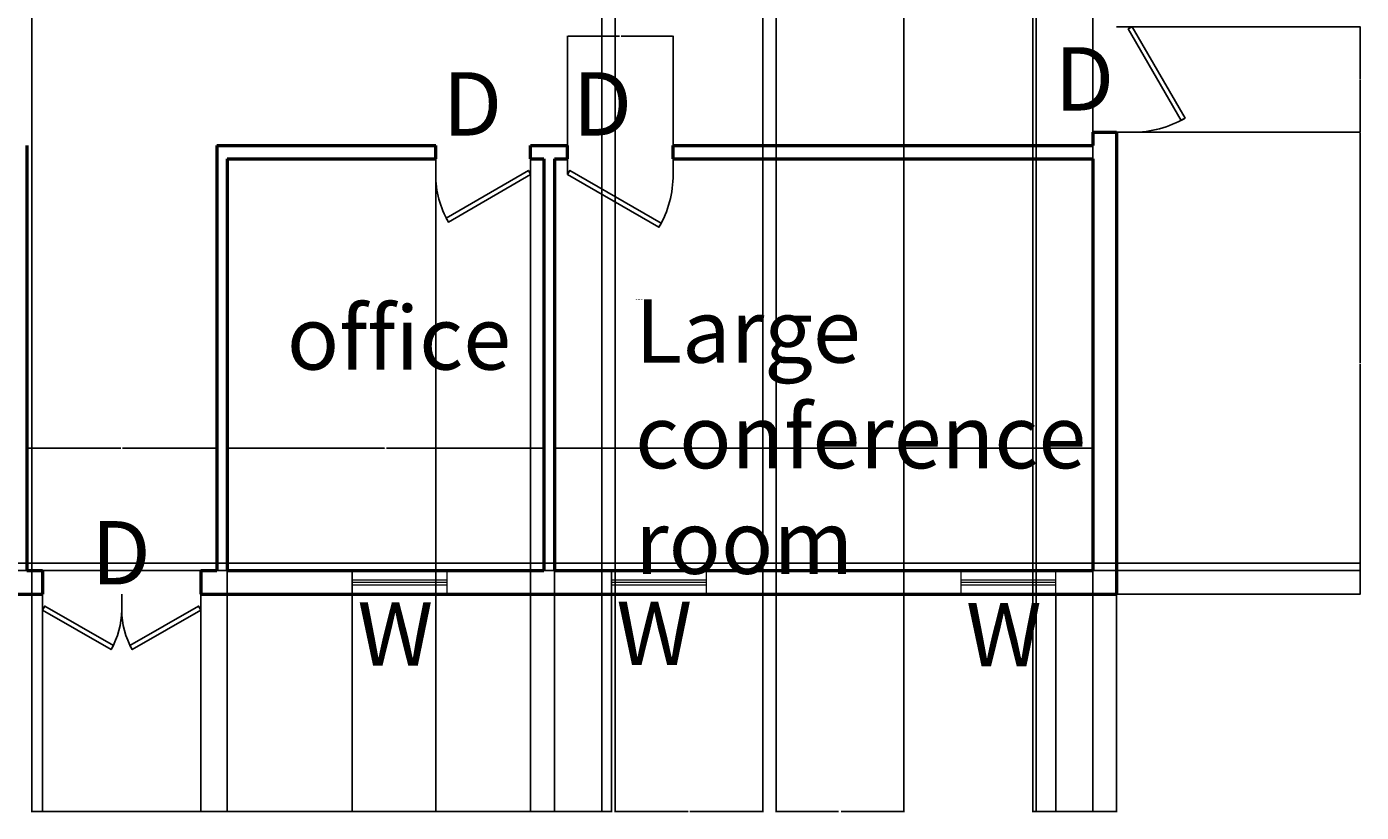
# Model space of a CAD drawing. Units: inches. Extents: x -84 to 931, y 65 to 668.
# Tile 3 of 5: x 426 to 931, y 65 to 363. Entities that reach past the tile are written whole.
import ezdxf

# ---------------------------------------------------------------- set-up
doc = ezdxf.new("R2010")
doc.units = ezdxf.units.IN
doc.header["$MEASUREMENT"] = 0
for name, color, linetype, lineweight in [('A-ANNO-DIMS', 2, 'Continuous', 18), ('A-ANNO-TEXT', 7, 'Continuous', 18), ('A-AREA-IDEN', 7, 'Continuous', 25), ('A-DOOR', 4, 'Continuous', 25), ('A-GLAZ', 4, 'Continuous', 18), ('A-WALL', 7, 'Continuous', 50)]:
    doc.layers.add(name, color=color, linetype=linetype, lineweight=lineweight)
doc.styles.get("Standard").update_dxf_attribs({"font": 'arial.ttf'})
doc.dimstyles.get("Standard").update_dxf_attribs({"dimtxt": 0.18, "dimasz": 0.18, "dimexe": 0.18, "dimexo": 0.0625, "dimgap": 0.09, "dimtad": 0, "dimtih": 1, "dimtoh": 1, "dimdec": 0, "dimzin": 0, "dimdsep": 46, "dimlunit": 3, "dimtxsty": 'Standard', "dimcen": 0.09, "dimadec": 0, "dimazin": 0, "dimtfac": 1, "dimtdec": 0, "dimtofl": 0, "dimtmove": 0, "dimatfit": 3, "dimfxl": 1, "dimtolj": 1, "dimtzin": 0, "dimarcsym": 0})

# ---------------------------------------------------------------- blocks, each defined once
blk = doc.blocks.new('*U7')
for p, q in [((0, 0), (0, 6)), ((40, 0), (40, 6))]:
    blk.add_line(p, q)
blk.add_lwpolyline([(0, 0), (34.64, -20), (35.52, -18.48), (0.88, 1.52)], close=True)
blk.add_arc((0, 0), 40, 330, 360)
blk = doc.blocks.new('*U8')
for p, q in [((-36, 0), (-36, 6)), ((0, 0), (0, 6))]:
    blk.add_line(p, q)
blk.add_lwpolyline([(0, 0), (-31.18, -18), (-32.05, -16.48), (-0.88, 1.52)], close=True)
blk.add_arc((0, 0), 36, 180, 210)
blk = doc.blocks.new('*U12')
for p, q in [((0, 0), (0, 6)), ((30, 0), (30, 6))]:
    blk.add_line(p, q)
blk.add_lwpolyline([(0, 0), (25.98, -15), (26.86, -13.48), (0.87, 1.52)], close=True)
blk.add_arc((0, 0), 30, 330, 0)
blk = doc.blocks.new('*U13')
for p, q in [((-40, 0), (-40, 6)), ((0, 0), (0, 6))]:
    blk.add_line(p, q)
blk.add_lwpolyline([(0, 0), (-34.64, -20), (-35.52, -18.48), (-0.87, 1.52)], close=True)
blk.add_arc((0, 0), 40, 180, 210)
blk = doc.blocks.new('WIN-36IN')
for p, q in [((3.5, 0), (3.5, 36)), ((4.5, 0), (4.5, 36)), ((5.5, 0), (5.5, 36))]:
    blk.add_line(p, q)
blk.add_lwpolyline([(0, 36), (0, 0), (9, 0), (9, 36)], close=True)
blk = doc.blocks.new('*D38')
at = {"layer": 'A-ANNO-DIMS', "color": 0, "lineweight": -2, "transparency": 16777216}
for p, q in [((427.53, 594.45), (427.53, 64.99)), ((643.53, 594.45), (643.53, 64.99)), ((427.71, 65.17), (535.14, 65.17)), ((643.35, 65.17), (535.92, 65.17))]:
    blk.add_line(p, q, dxfattribs=at)
at = {"layer": 'A-ANNO-DIMS', "color": 0, "transparency": 16777216}
for points in [[(427.71, 65.2), (427.71, 65.14), (427.53, 65.17)], [(643.35, 65.2), (643.35, 65.14), (643.53, 65.17)]]:
    blk.add_solid(points, dxfattribs=at)
at = {"layer": 'Defpoints', "color": 0, "transparency": 16777216}
for p in [(427.53, 594.52), (643.53, 594.52), (643.53, 65.17)]:
    blk.add_point(p, dxfattribs=at)
at = {"layer": 'A-ANNO-DIMS', "color": 0, "transparency": 16777216, "insert": (535.53, 65.17), "char_height": 0.18, "attachment_point": 5}
blk.add_mtext('\\A1;18\'-0"', dxfattribs=at)
blk = doc.blocks.new('*D39')
at = {"layer": 'A-ANNO-DIMS', "color": 0, "lineweight": -2, "transparency": 16777216}
for p, q in [((648.53, 594.45), (648.53, 64.99)), ((704.53, 594.45), (704.53, 64.99)), ((648.71, 65.17), (676.2, 65.17)), ((704.35, 65.17), (676.86, 65.17))]:
    blk.add_line(p, q, dxfattribs=at)
at = {"layer": 'A-ANNO-DIMS', "color": 0, "transparency": 16777216}
for points in [[(648.71, 65.2), (648.71, 65.14), (648.53, 65.17)], [(704.35, 65.2), (704.35, 65.14), (704.53, 65.17)]]:
    blk.add_solid(points, dxfattribs=at)
at = {"layer": 'Defpoints', "color": 0, "transparency": 16777216}
for p in [(648.53, 594.52), (704.53, 594.52), (704.53, 65.17)]:
    blk.add_point(p, dxfattribs=at)
at = {"layer": 'A-ANNO-DIMS', "color": 0, "transparency": 16777216, "insert": (676.53, 65.17), "char_height": 0.18, "attachment_point": 5}
blk.add_mtext('\\A1;4\'-8"', dxfattribs=at)
blk = doc.blocks.new('*D43')
at = {"layer": 'A-ANNO-DIMS', "color": 0, "lineweight": -2, "transparency": 16777216}
for p, q in [((425.53, 156.58), (425.53, 203.05)), ((425.71, 202.87), (461.2, 202.87)), ((497.35, 202.87), (461.86, 202.87)), ((497.53, 156.58), (497.53, 203.05))]:
    blk.add_line(p, q, dxfattribs=at)
at = {"layer": 'A-ANNO-DIMS', "color": 0, "transparency": 16777216}
for points in [[(425.71, 202.9), (425.71, 202.84), (425.53, 202.87)], [(497.35, 202.9), (497.35, 202.84), (497.53, 202.87)]]:
    blk.add_solid(points, dxfattribs=at)
at = {"layer": 'Defpoints', "color": 0, "transparency": 16777216}
for p in [(497.53, 202.87), (425.53, 156.52), (497.53, 156.52)]:
    blk.add_point(p, dxfattribs=at)
at = {"layer": 'A-ANNO-DIMS', "color": 0, "transparency": 16777216, "insert": (461.53, 202.87), "char_height": 0.18, "attachment_point": 5}
blk.add_mtext('\\A1;6\'-0"', dxfattribs=at)
blk = doc.blocks.new('*D44')
at = {"layer": 'A-ANNO-DIMS', "color": 0, "lineweight": -2, "transparency": 16777216}
for p, q in [((501.53, 156.58), (501.53, 203.05)), ((501.71, 202.87), (561.14, 202.87)), ((621.35, 202.87), (561.92, 202.87)), ((621.53, 156.58), (621.53, 203.05))]:
    blk.add_line(p, q, dxfattribs=at)
at = {"layer": 'A-ANNO-DIMS', "color": 0, "transparency": 16777216}
for points in [[(501.71, 202.9), (501.71, 202.84), (501.53, 202.87)], [(621.35, 202.9), (621.35, 202.84), (621.53, 202.87)]]:
    blk.add_solid(points, dxfattribs=at)
at = {"layer": 'Defpoints', "color": 0, "transparency": 16777216}
for p in [(621.53, 202.87), (501.53, 156.52), (621.53, 156.52)]:
    blk.add_point(p, dxfattribs=at)
at = {"layer": 'A-ANNO-DIMS', "color": 0, "transparency": 16777216, "insert": (561.53, 202.87), "char_height": 0.18, "attachment_point": 5}
blk.add_mtext('\\A1;10\'-0"', dxfattribs=at)
blk = doc.blocks.new('*D45')
at = {"layer": 'A-ANNO-DIMS', "color": 0, "lineweight": -2, "transparency": 16777216}
for p, q in [((625.53, 156.58), (625.53, 203.05)), ((625.71, 202.87), (727.14, 202.87)), ((829.35, 202.87), (727.92, 202.87)), ((829.53, 156.58), (829.53, 203.05))]:
    blk.add_line(p, q, dxfattribs=at)
at = {"layer": 'A-ANNO-DIMS', "color": 0, "transparency": 16777216}
for points in [[(625.71, 202.9), (625.71, 202.84), (625.53, 202.87)], [(829.35, 202.9), (829.35, 202.84), (829.53, 202.87)]]:
    blk.add_solid(points, dxfattribs=at)
at = {"layer": 'Defpoints', "color": 0, "transparency": 16777216}
for p in [(829.53, 202.87), (625.53, 156.52), (829.53, 156.52)]:
    blk.add_point(p, dxfattribs=at)
at = {"layer": 'A-ANNO-DIMS', "color": 0, "transparency": 16777216, "insert": (727.53, 202.87), "char_height": 0.18, "attachment_point": 5}
blk.add_mtext('\\A1;17\'-0"', dxfattribs=at)
blk = doc.blocks.new('*D51')
at = {"layer": 'A-ANNO-DIMS', "color": 0, "lineweight": -2, "transparency": 16777216}
for p, q in [((431.53, 147.45), (431.53, 64.99)), ((491.53, 147.45), (491.53, 64.99)), ((431.71, 65.17), (461.2, 65.17)), ((491.35, 65.17), (461.86, 65.17))]:
    blk.add_line(p, q, dxfattribs=at)
at = {"layer": 'A-ANNO-DIMS', "color": 0, "transparency": 16777216}
for points in [[(431.71, 65.2), (431.71, 65.14), (431.53, 65.17)], [(491.35, 65.2), (491.35, 65.14), (491.53, 65.17)]]:
    blk.add_solid(points, dxfattribs=at)
at = {"layer": 'Defpoints', "color": 0, "transparency": 16777216}
for p in [(431.53, 147.52), (491.53, 147.52), (491.53, 65.17)]:
    blk.add_point(p, dxfattribs=at)
at = {"layer": 'A-ANNO-DIMS', "color": 0, "transparency": 16777216, "insert": (461.53, 65.17), "char_height": 0.18, "attachment_point": 5}
blk.add_mtext('\\A1;5\'-0"', dxfattribs=at)
blk = doc.blocks.new('*D53')
at = {"layer": 'A-ANNO-DIMS', "color": 0, "lineweight": -2, "transparency": 16777216}
for p, q in [((838.59, 362.52), (931.06, 362.52)), ((930.88, 362.34), (930.88, 342.7)), ((930.88, 322.7), (930.88, 342.33)), ((838.59, 322.52), (931.06, 322.52))]:
    blk.add_line(p, q, dxfattribs=at)
at = {"layer": 'A-ANNO-DIMS', "color": 0, "transparency": 16777216}
for points in [[(930.85, 362.34), (930.91, 362.34), (930.88, 362.52)], [(930.85, 322.7), (930.91, 322.7), (930.88, 322.52)]]:
    blk.add_solid(points, dxfattribs=at)
at = {"layer": 'Defpoints', "color": 0, "transparency": 16777216}
for p in [(838.53, 362.52), (930.88, 362.52), (838.53, 322.52)]:
    blk.add_point(p, dxfattribs=at)
at = {"layer": 'A-ANNO-DIMS', "color": 0, "transparency": 16777216, "insert": (930.88, 342.52), "char_height": 0.18, "attachment_point": 5}
blk.add_mtext('\\A1;3\'-4"', dxfattribs=at)
blk = doc.blocks.new('*D58')
at = {"layer": 'A-ANNO-DIMS', "color": 0, "lineweight": -2, "transparency": 16777216}
for p, q in [((501.53, 156.45), (501.53, 64.99)), ((548.85, 156.45), (548.85, 64.99)), ((501.71, 65.17), (524.58, 65.17)), ((548.67, 65.17), (525.8, 65.17))]:
    blk.add_line(p, q, dxfattribs=at)
at = {"layer": 'A-ANNO-DIMS', "color": 0, "transparency": 16777216}
for points in [[(501.71, 65.2), (501.71, 65.14), (501.53, 65.17)], [(548.67, 65.2), (548.67, 65.14), (548.85, 65.17)]]:
    blk.add_solid(points, dxfattribs=at)
at = {"layer": 'Defpoints', "color": 0, "transparency": 16777216}
for p in [(501.53, 156.52), (548.85, 156.52), (548.85, 65.17)]:
    blk.add_point(p, dxfattribs=at)
at = {"layer": 'A-ANNO-DIMS', "color": 0, "transparency": 16777216, "insert": (525.19, 65.17), "char_height": 0.18, "attachment_point": 5}
blk.add_mtext('\\A1;3\'-11 1/2"', dxfattribs=at)
blk = doc.blocks.new('*D59')
at = {"layer": 'A-ANNO-DIMS', "color": 0, "lineweight": -2, "transparency": 16777216}
for p, q in [((625.53, 156.45), (625.53, 64.99)), ((647.22, 156.45), (647.22, 64.99)), ((625.71, 65.17), (635.85, 65.17)), ((647.04, 65.17), (636.91, 65.17))]:
    blk.add_line(p, q, dxfattribs=at)
at = {"layer": 'A-ANNO-DIMS', "color": 0, "transparency": 16777216}
for points in [[(625.71, 65.2), (625.71, 65.14), (625.53, 65.17)], [(647.04, 65.2), (647.04, 65.14), (647.22, 65.17)]]:
    blk.add_solid(points, dxfattribs=at)
at = {"layer": 'Defpoints', "color": 0, "transparency": 16777216}
for p in [(625.53, 156.52), (647.22, 156.52), (647.22, 65.17)]:
    blk.add_point(p, dxfattribs=at)
at = {"layer": 'A-ANNO-DIMS', "color": 0, "transparency": 16777216, "insert": (636.38, 65.17), "char_height": 0.18, "attachment_point": 5}
blk.add_mtext('\\A1;1\'-9 1/2"', dxfattribs=at)
blk = doc.blocks.new('*D60')
at = {"layer": 'A-ANNO-DIMS', "color": 0, "lineweight": -2, "transparency": 16777216}
for p, q in [((815.62, 147.45), (815.62, 64.99)), ((838.53, 147.45), (838.53, 64.99)), ((815.8, 65.17), (826.69, 65.17)), ((838.35, 65.17), (827.47, 65.17))]:
    blk.add_line(p, q, dxfattribs=at)
at = {"layer": 'A-ANNO-DIMS', "color": 0, "transparency": 16777216}
for points in [[(815.8, 65.2), (815.8, 65.14), (815.62, 65.17)], [(838.35, 65.2), (838.35, 65.14), (838.53, 65.17)]]:
    blk.add_solid(points, dxfattribs=at)
at = {"layer": 'Defpoints', "color": 0, "transparency": 16777216}
for p in [(815.62, 147.52), (838.53, 147.52), (838.53, 65.17)]:
    blk.add_point(p, dxfattribs=at)
at = {"layer": 'A-ANNO-DIMS', "color": 0, "transparency": 16777216, "insert": (827.08, 65.17), "char_height": 0.18, "attachment_point": 5}
blk.add_mtext('\\A1;1\'-11"', dxfattribs=at)
blk = doc.blocks.new('*D63')
at = {"layer": 'A-ANNO-DIMS', "color": 0, "lineweight": -2, "transparency": 16777216}
for p, q in [((580.53, 317.45), (580.53, 64.99)), ((616.53, 317.45), (616.53, 64.99)), ((580.71, 65.17), (598.2, 65.17)), ((616.35, 65.17), (598.86, 65.17))]:
    blk.add_line(p, q, dxfattribs=at)
at = {"layer": 'A-ANNO-DIMS', "color": 0, "transparency": 16777216}
for points in [[(580.71, 65.2), (580.71, 65.14), (580.53, 65.17)], [(616.35, 65.2), (616.35, 65.14), (616.53, 65.17)]]:
    blk.add_solid(points, dxfattribs=at)
at = {"layer": 'Defpoints', "color": 0, "transparency": 16777216}
for p in [(580.53, 317.52), (616.53, 317.52), (616.53, 65.17)]:
    blk.add_point(p, dxfattribs=at)
at = {"layer": 'A-ANNO-DIMS', "color": 0, "transparency": 16777216, "insert": (598.53, 65.17), "char_height": 0.18, "attachment_point": 5}
blk.add_mtext('\\A1;3\'-0"', dxfattribs=at)
blk = doc.blocks.new('*D64')
at = {"layer": 'A-ANNO-DIMS', "color": 0, "lineweight": -2, "transparency": 16777216}
for p, q in [((838.59, 322.52), (931.06, 322.52)), ((930.88, 322.34), (930.88, 235.2)), ((930.88, 147.7), (930.88, 234.84)), ((838.59, 147.52), (931.06, 147.52))]:
    blk.add_line(p, q, dxfattribs=at)
at = {"layer": 'A-ANNO-DIMS', "color": 0, "transparency": 16777216}
for points in [[(930.85, 322.34), (930.91, 322.34), (930.88, 322.52)], [(930.85, 147.7), (930.91, 147.7), (930.88, 147.52)]]:
    blk.add_solid(points, dxfattribs=at)
at = {"layer": 'Defpoints', "color": 0, "transparency": 16777216}
for p in [(838.53, 322.52), (930.88, 322.52), (838.53, 147.52)]:
    blk.add_point(p, dxfattribs=at)
at = {"layer": 'A-ANNO-DIMS', "color": 0, "transparency": 16777216, "insert": (930.88, 235.02), "char_height": 0.18, "attachment_point": 5}
blk.add_mtext('\\A1;14\'-7"', dxfattribs=at)
blk = doc.blocks.new('*D68')
at = {"layer": 'A-ANNO-DIMS', "color": 0, "lineweight": -2, "transparency": 16777216}
for p, q in [((709.53, 450.45), (709.53, 64.99)), ((757.92, 450.45), (757.92, 64.99)), ((709.71, 65.17), (733.18, 65.17)), ((757.74, 65.17), (734.27, 65.17))]:
    blk.add_line(p, q, dxfattribs=at)
at = {"layer": 'A-ANNO-DIMS', "color": 0, "transparency": 16777216}
for points in [[(709.71, 65.2), (709.71, 65.14), (709.53, 65.17)], [(757.74, 65.2), (757.74, 65.14), (757.92, 65.17)]]:
    blk.add_solid(points, dxfattribs=at)
at = {"layer": 'Defpoints', "color": 0, "transparency": 16777216}
for p in [(709.53, 450.52), (757.92, 450.52), (757.92, 65.17)]:
    blk.add_point(p, dxfattribs=at)
at = {"layer": 'A-ANNO-DIMS', "color": 0, "transparency": 16777216, "insert": (733.73, 65.17), "char_height": 0.18, "attachment_point": 5}
blk.add_mtext('\\A1;4\'-0 1/2"', dxfattribs=at)
blk = doc.blocks.new('*D78')
at = {"layer": 'A-ANNO-DIMS', "color": 0, "lineweight": -2, "transparency": 16777216}
for p, q in [((182.71, 159.24), (931.06, 159.24)), ((930.88, 159.06), (930.88, 158.06)), ((930.88, 156.7), (930.88, 157.69)), ((217.59, 156.52), (931.06, 156.52))]:
    blk.add_line(p, q, dxfattribs=at)
at = {"layer": 'A-ANNO-DIMS', "color": 0, "transparency": 16777216}
for points in [[(930.85, 159.06), (930.91, 159.06), (930.88, 159.24)], [(930.85, 156.7), (930.91, 156.7), (930.88, 156.52)]]:
    blk.add_solid(points, dxfattribs=at)
at = {"layer": 'Defpoints', "color": 0, "transparency": 16777216}
for p in [(182.65, 159.24), (217.53, 156.52), (930.88, 156.52)]:
    blk.add_point(p, dxfattribs=at)
at = {"layer": 'A-ANNO-DIMS', "color": 0, "transparency": 16777216, "insert": (930.88, 157.88), "char_height": 0.18, "attachment_point": 5}
blk.add_mtext('\\A1;0\'-2 1/2"', dxfattribs=at)
blk = doc.blocks.new('*D87')
at = {"layer": 'A-ANNO-DIMS', "color": 0, "lineweight": -2, "transparency": 16777216}
for p, q in [((630.53, 312.58), (630.53, 359.05)), ((630.71, 358.87), (650.2, 358.87)), ((670.35, 358.87), (650.86, 358.87)), ((670.53, 312.58), (670.53, 359.05))]:
    blk.add_line(p, q, dxfattribs=at)
at = {"layer": 'A-ANNO-DIMS', "color": 0, "transparency": 16777216}
for points in [[(630.71, 358.9), (630.71, 358.84), (630.53, 358.87)], [(670.35, 358.9), (670.35, 358.84), (670.53, 358.87)]]:
    blk.add_solid(points, dxfattribs=at)
at = {"layer": 'Defpoints', "color": 0, "transparency": 16777216}
for p in [(670.53, 358.87), (630.53, 312.52), (670.53, 312.52)]:
    blk.add_point(p, dxfattribs=at)
at = {"layer": 'A-ANNO-DIMS', "color": 0, "transparency": 16777216, "insert": (650.53, 358.87), "char_height": 0.18, "attachment_point": 5}
blk.add_mtext('\\A1;3\'-4"', dxfattribs=at)
blk = doc.blocks.new('*D89')
at = {"layer": 'A-ANNO-DIMS', "color": 0, "lineweight": -2, "transparency": 16777216}
for p, q in [((808.07, 528.04), (808.07, 64.99)), ((829.53, 524.45), (829.53, 64.99)), ((808.25, 65.17), (818.27, 65.17)), ((829.35, 65.17), (819.33, 65.17))]:
    blk.add_line(p, q, dxfattribs=at)
at = {"layer": 'A-ANNO-DIMS', "color": 0, "transparency": 16777216}
for points in [[(808.25, 65.2), (808.25, 65.14), (808.07, 65.17)], [(829.35, 65.2), (829.35, 65.14), (829.53, 65.17)]]:
    blk.add_solid(points, dxfattribs=at)
at = {"layer": 'Defpoints', "color": 0, "transparency": 16777216}
for p in [(808.07, 528.1), (829.53, 524.52), (829.53, 65.17)]:
    blk.add_point(p, dxfattribs=at)
at = {"layer": 'A-ANNO-DIMS', "color": 0, "transparency": 16777216, "insert": (818.8, 65.17), "char_height": 0.18, "attachment_point": 5}
blk.add_mtext('\\A1;1\'-9 1/2"', dxfattribs=at)
blk = doc.blocks.new('*D90')
at = {"layer": 'A-ANNO-DIMS', "color": 0, "lineweight": -2, "transparency": 16777216}
for p, q in [((806.83, 455.7), (806.83, 64.99)), ((829.53, 450.45), (829.53, 64.99)), ((807.01, 65.17), (817.58, 65.17)), ((829.35, 65.17), (818.78, 65.17))]:
    blk.add_line(p, q, dxfattribs=at)
at = {"layer": 'A-ANNO-DIMS', "color": 0, "transparency": 16777216}
for points in [[(807.01, 65.2), (807.01, 65.14), (806.83, 65.17)], [(829.35, 65.2), (829.35, 65.14), (829.53, 65.17)]]:
    blk.add_solid(points, dxfattribs=at)
at = {"layer": 'Defpoints', "color": 0, "transparency": 16777216}
for p in [(806.83, 455.77), (829.53, 450.52), (829.53, 65.17)]:
    blk.add_point(p, dxfattribs=at)
at = {"layer": 'A-ANNO-DIMS', "color": 0, "transparency": 16777216, "insert": (818.18, 65.17), "char_height": 0.18, "attachment_point": 5}
blk.add_mtext('\\A1;1\'-10 1/2"', dxfattribs=at)

msp = doc.modelspace()

# ---------------------------------------------------------------- linework, layer by layer
at = {"layer": 'A-WALL'}
for p, q in [((829.53, 322.52), (838.53, 322.52)), ((829.53, 322.52), (829.53, 317.52)), ((838.53, 322.52), (838.53, 147.52)), ((425.53, 317.52), (425.53, 156.52)), ((497.53, 317.52), (497.53, 156.52)), ((497.53, 317.52), (580.53, 317.52)), ((580.53, 312.52), (580.53, 317.52)), ((616.53, 312.52), (616.53, 317.52)), ((616.53, 317.52), (630.53, 317.52)), ((630.53, 312.52), (630.53, 317.52)), ((670.53, 312.52), (670.53, 317.52)), ((670.53, 317.52), (829.53, 317.52)), ((501.53, 312.52), (501.53, 156.52)), ((501.53, 312.52), (580.53, 312.52)), ((616.53, 312.52), (621.53, 312.52)), ((621.53, 312.52), (621.53, 156.52)), ((625.53, 312.52), (625.53, 156.52)), ((625.53, 312.52), (630.53, 312.52)), ((670.53, 312.52), (829.53, 312.52)), ((829.53, 312.52), (829.53, 156.52)), ((425.53, 156.52), (431.53, 156.52)), ((431.53, 156.52), (431.53, 147.52)), ((491.53, 156.52), (491.53, 147.52)), ((491.53, 156.52), (497.53, 156.52)), ((501.53, 156.52), (621.53, 156.52)), ((625.53, 156.52), (829.53, 156.52)), ((0.53, 147.52), (431.53, 147.52)), ((491.53, 147.52), (838.53, 147.52))]:
    msp.add_line(p, q, dxfattribs=at)

# ---------------------------------------------------------------- block references
at = {"layer": 'A-DOOR', "rotation": 90}
msp.add_blockref('*U13', (844.53, 362.52), dxfattribs=at)
at = {"layer": 'A-DOOR'}
for name, p in [('*U8', (616.53, 306.52)), ('*U7', (630.53, 306.52)), ('*U12', (431.53, 141.52))]:
    msp.add_blockref(name, p, dxfattribs=at)
at = {"layer": 'A-DOOR', "xscale": -1}
msp.add_blockref('*U12', (491.53, 141.52), dxfattribs=at)
at = {"layer": 'A-GLAZ'}
for p, rotation in [((548.85, 156.52), 270.0000000000002), ((647.22, 156.52), 270.0000000000001), ((779.62, 156.52), 270.0000000000001)]:
    msp.add_blockref('WIN-36IN', p, dxfattribs=dict(at, rotation=rotation))

# ---------------------------------------------------------------- texts
at = {"layer": 'A-ANNO-TEXT', "char_height": 24, "attachment_point": 1}
for s, width, insert in [('D', 21.9508, (815.14, 354.75)), ('D', 21.9508, (583.21, 345.27)), ('D', 21.9508, (632.43, 345.27)), ('D', 21.9508, (450.01, 175.21)), ('W', 20.4711, (550.86, 144.5)), ('W', 20.4711, (649.01, 144.7)), ('W', 20.4711, (781.49, 144.23))]:
    msp.add_mtext_dynamic_manual_height_columns(s, width=width, gutter_width=1, heights=[0], dxfattribs=dict(at, insert=insert))
at = {"layer": 'A-AREA-IDEN', "attachment_point": 1}
for s, width, insert, char_height in [('office', 70.4822, (524.14, 256.61), 24), ('Large conference room', 129.1102, (656.12, 259.23), 0.2), ('Large conference room', 131.8349, (656.12, 259.23), 24)]:
    msp.add_mtext_dynamic_manual_height_columns(s, width=width, gutter_width=1, heights=[0], dxfattribs=dict(at, insert=insert, char_height=char_height))

# ---------------------------------------------------------------- dimensions: what is measured, and where the dimension line sits
at = {"layer": 'A-ANNO-DIMS'}
for base, p1, p2, picture, middle in [((643.53, 65.17), (427.53, 594.52), (643.53, 594.52), '*D38', (535.53, 65.17)), ((704.53, 65.17), (648.53, 594.52), (704.53, 594.52), '*D39', (676.53, 65.17)), ((829.53, 65.17), (808.07, 528.1), (829.53, 524.52), '*D89', (818.8, 65.17)), ((829.53, 65.17), (806.83, 455.77), (829.53, 450.52), '*D90', (818.18, 65.17)), ((757.92, 65.17), (709.53, 450.52), (757.92, 450.52), '*D68', (733.73, 65.17)), ((670.53, 358.87), (630.53, 312.52), (670.53, 312.52), '*D87', (650.53, 358.87)), ((616.53, 65.17), (580.53, 317.52), (616.53, 317.52), '*D63', (598.53, 65.17)), ((497.53, 202.87), (425.53, 156.52), (497.53, 156.52), '*D43', (461.53, 202.87)), ((621.53, 202.87), (501.53, 156.52), (621.53, 156.52), '*D44', (561.53, 202.87)), ((829.53, 202.87), (625.53, 156.52), (829.53, 156.52), '*D45', (727.53, 202.87)), ((548.85, 65.17), (501.53, 156.52), (548.85, 156.52), '*D58', (525.19, 65.17)), ((647.22, 65.17), (625.53, 156.52), (647.22, 156.52), '*D59', (636.38, 65.17)), ((491.53, 65.17), (431.53, 147.52), (491.53, 147.52), '*D51', (461.53, 65.17)), ((838.53, 65.17), (815.62, 147.52), (838.53, 147.52), '*D60', (827.08, 65.17))]:
    dim = msp.add_linear_dim(base=base, p1=p1, p2=p2, dimstyle='Standard', override={"dimdec": 1, "dimlfac": 1, "dimrnd": 0, "dimzin": 1, "dimdsep": 46, "dimlunit": 4, "dimfrac": 2}, dxfattribs=at)
    dim.commit()
    dim.dimension.update_dxf_attribs({"geometry": picture, "text_midpoint": middle})
for base, p1, p2, picture, middle in [((930.88, 362.52), (838.53, 322.52), (838.53, 362.52), '*D53', (930.88, 342.52)), ((930.88, 322.52), (838.53, 147.52), (838.53, 322.52), '*D64', (930.88, 235.02)), ((930.88, 156.52), (182.65, 159.24), (217.53, 156.52), '*D78', (930.88, 157.88))]:
    dim = msp.add_linear_dim(base=base, p1=p1, p2=p2, angle=90, dimstyle='Standard', override={"dimdec": 1, "dimlfac": 1, "dimrnd": 0, "dimzin": 1, "dimdsep": 46, "dimlunit": 4, "dimfrac": 2}, dxfattribs=at)
    dim.commit()
    dim.dimension.update_dxf_attribs({"geometry": picture, "text_midpoint": middle})

doc.saveas('drawing.dxf')
